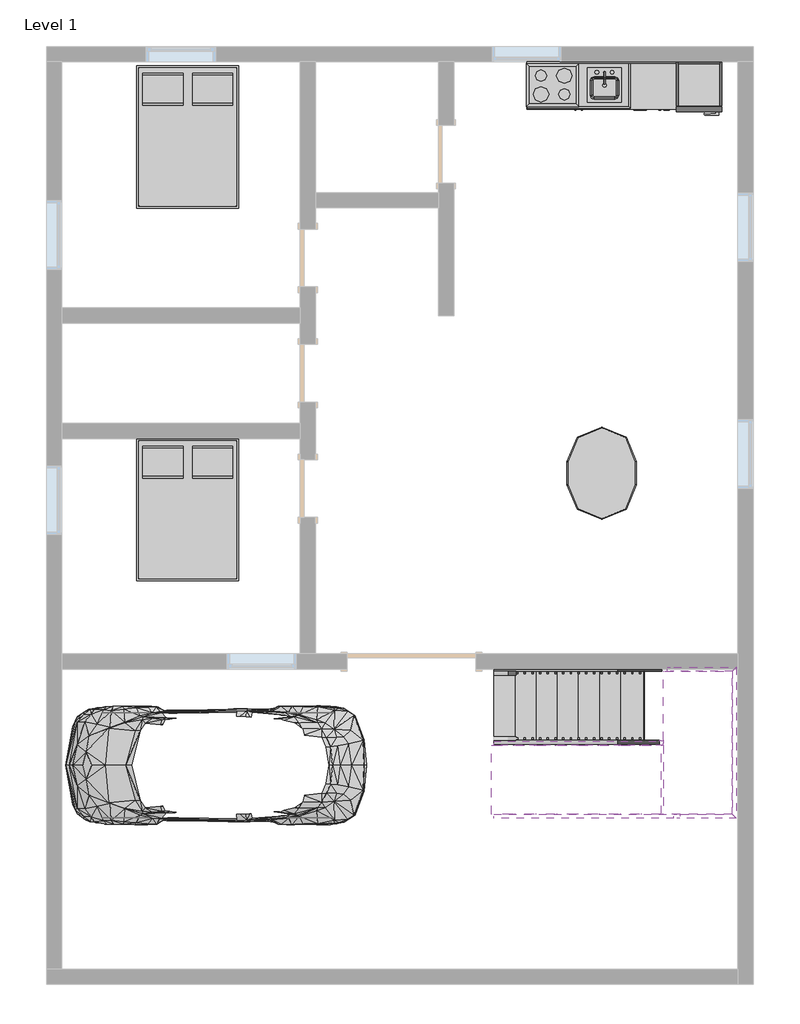
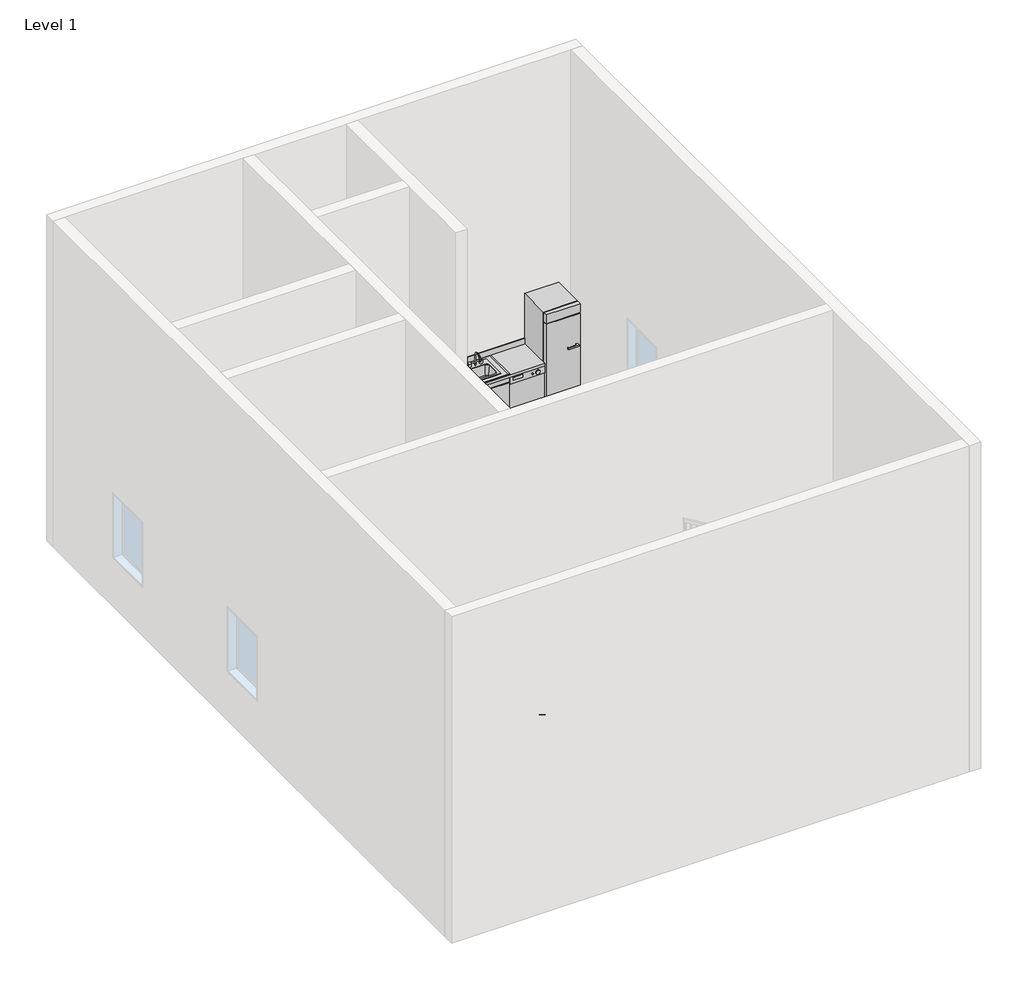
# One storey, part 2 of 2: 8 members, 5 proxies, 4 furniture elements, 2 stair flights, 1 flow terminal, 1 railing, 1 slab.
"""IFC4 building model written with IfcOpenShell, lengths in millimetres."""

from ifc_helpers import new_model, si_unit, frame, origin, place, context, project, spatial, polyline, outline, extrude, faceted_brep, transform, mapped, element, save
from components import m_cook_top_4_unit2_0615_x_500mm_249f3515, m_dishwasher_610_x_610_x_875mm_54ecfc4c, m_kitchenette_medium_1372mm_e05c6bec, m_rpc_beetle_m_rpc_beetle_aa710b07, m_refrigerator_600_x_660mm_a466bf94, m_sink_kitchen_island_450_x_450mm_f969cf2d, m_bed_box_1346_x_1880mm_double_b32eb57e, m_counter_top_w_sink_hole_600mm_depth_0a237b63, m_table_dining_oval_0915_x_1220mm_c3de6a6b, non_monolithic_landing_275f9134, stair_flight_1fa62499, stair_flight_e850d810

model = new_model("IFC4")

# Units and contexts
model_context = context("Model", 3, world=origin())
ifc_project = project(units=[si_unit("LENGTHUNIT", "METRE", prefix="MILLI")], contexts=[model_context])

# Site, building, storey
site = spatial("IfcSite", under=ifc_project)
building = spatial("IfcBuilding", under=site)
storey = spatial("IfcBuildingStorey", under=building, Name="Level 1", Elevation=0.0)

# Proxies
placement = place(None, origin())
m_cook_top_4_unit2_0615_x_500mm_shape = m_cook_top_4_unit2_0615_x_500mm_249f3515(model_context)
element("IfcBuildingElementProxy", 1, Name="M_Cook Top-4 Unit2 : 0615 x 500mm", ObjectType="M_Cook Top-4 Unit2 : 0615 x 500mm", at=placement, inside=storey, context=model_context, shape_type="MappedRepresentation", body=[
    mapped(m_cook_top_4_unit2_0615_x_500mm_shape, transform((-3150.6851125, 9903.2979873, 0.0), x_axis=(1.0, 0.0, 0.0), y_axis=(0.0, 1.0, 0.0), z_axis=(0.0, 0.0, 1.0))),
])
m_dishwasher_610_x_610_x_875mm_shape = m_dishwasher_610_x_610_x_875mm_54ecfc4c(model_context)
element("IfcBuildingElementProxy", 2, Name="M_Dishwasher : 610 x 610 x 875mm", ObjectType="M_Dishwasher : 610 x 610 x 875mm", at=placement, inside=storey, context=model_context, shape_type="MappedRepresentation", body=[
    mapped(m_dishwasher_610_x_610_x_875mm_shape, transform((-2201.202581, 9636.6484225, 0.0), x_axis=(1.0, 0.0, 0.0), y_axis=(0.0, 1.0, 0.0), z_axis=(0.0, 0.0, 1.0))),
])
m_kitchenette_medium_1372mm_shape = m_kitchenette_medium_1372mm_e05c6bec(model_context)
element("IfcBuildingElementProxy", 3, Name="M_Kitchenette - Medium : 1372mm", ObjectType="M_Kitchenette - Medium : 1372mm", at=placement, inside=storey, context=model_context, shape_type="MappedRepresentation", body=[
    mapped(m_kitchenette_medium_1372mm_shape, transform((-2826.4228174, 10208.2979873, 0.0), x_axis=(1.0, 0.0, 0.0), y_axis=(0.0, 1.0, 0.0), z_axis=(0.0, 0.0, 1.0))),
])
m_rpc_beetle_m_rpc_beetle_shape = m_rpc_beetle_m_rpc_beetle_aa710b07(model_context)
element("IfcBuildingElementProxy", 4, Name="M_RPC Beetle : M_RPC Beetle", ObjectType="M_RPC Beetle : M_RPC Beetle", at=placement, inside=storey, context=model_context, shape_type="MappedRepresentation", body=[
    mapped(m_rpc_beetle_m_rpc_beetle_shape, transform((-6363.8851125, 911.8979873, 0.0), x_axis=(0.0, 1.0000000000000002, 0.0), y_axis=(-1.0000000000000002, 0.0, 0.0), z_axis=(0.0, 0.0, 1.0))),
])
m_refrigerator_600_x_660mm_shape = m_refrigerator_600_x_660mm_a466bf94(model_context)
element("IfcBuildingElementProxy", 5, Name="M_Refrigerator : 600 x 660mm", ObjectType="M_Refrigerator : 600 x 660mm", at=placement, inside=storey, context=model_context, shape_type="MappedRepresentation", body=[
    mapped(m_refrigerator_600_x_660mm_shape, transform((-1159.8839698, 9912.0828971, 0.0), x_axis=(1.0, 0.0, 0.0), y_axis=(0.0, 1.0, 0.0), z_axis=(0.0, 0.0, 1.0))),
])

# Flow terminal
m_sink_kitchen_island_450_x_450mm_shape = m_sink_kitchen_island_450_x_450mm_f969cf2d(model_context)
element("IfcFlowTerminal", 6, ObjectType="M_Sink Kitchen-Island : 450 x 450mm", at=placement, inside=storey, context=model_context, shape_type="MappedRepresentation", body=[
    mapped(m_sink_kitchen_island_450_x_450mm_shape, transform((-2480.374353, 9900.9525861, 0.0), x_axis=(1.0, 0.0, 0.0), y_axis=(0.0, 1.0, 0.0), z_axis=(0.0, 0.0, 1.0))),
])

# Furniture
m_bed_box_1346_x_1880mm_double_shape = m_bed_box_1346_x_1880mm_double_b32eb57e(model_context)
element("IfcFurniture", 7, ObjectType="M_Bed-Box : 1346 x 1880mm - Double", at=placement, inside=storey, context=model_context, shape_type="MappedRepresentation", body=[
    mapped(m_bed_box_1346_x_1880mm_double_shape, transform((-8315.8375715, 9452.3274955, 0.0), x_axis=(1.0, 0.0, 0.0), y_axis=(0.0, 1.0, 0.0), z_axis=(0.0, 0.0, 1.0))),
])
element("IfcFurniture", 8, ObjectType="M_Bed-Box : 1346 x 1880mm - Double", at=placement, inside=storey, context=model_context, shape_type="MappedRepresentation", body=[
    mapped(m_bed_box_1346_x_1880mm_double_shape, transform((-8315.8375715, 4524.3274955, 0.0), x_axis=(1.0, 0.0, 0.0), y_axis=(0.0, 1.0, 0.0), z_axis=(0.0, 0.0, 1.0))),
])
m_counter_top_w_sink_hole_600mm_depth_shape = m_counter_top_w_sink_hole_600mm_depth_0a237b63(model_context)
element("IfcFurniture", 9, ObjectType="M_Counter Top w Sink Hole : 600mm Depth", at=placement, inside=storey, context=model_context, shape_type="MappedRepresentation", body=[
    mapped(m_counter_top_w_sink_hole_600mm_depth_shape, transform((-2293.2228174, 10208.2979873, 0.0), x_axis=(1.0, 0.0, 0.0), y_axis=(0.0, 1.0, 0.0), z_axis=(0.0, 0.0, 1.0))),
])
m_table_dining_oval_0915_x_1220mm_shape = m_table_dining_oval_0915_x_1220mm_c3de6a6b(model_context)
element("IfcFurniture", 10, ObjectType="M_Table-Dining Oval : 0915 x 1220mm", at=placement, inside=storey, context=model_context, shape_type="MappedRepresentation", body=[
    mapped(m_table_dining_oval_0915_x_1220mm_shape, transform((-2860.4834731, 5174.2176594, 0.0), x_axis=(0.0, 1.0000000000000002, 0.0), y_axis=(-1.0000000000000002, 0.0, 0.0), z_axis=(0.0, 0.0, 1.0))),
])

# Members
element("IfcMember", 11, ObjectType="Stringer - 2\" Width", at=placement, inside=storey, context=model_context, shape_type="SweptSolid", body=[
    extrude(outline(polyline([(212.114512, -3925.4851125), (0.0, -3925.4851125), (0.0, -3687.3996007), (1295.4, -1549.9896007), (1600.2, -1635.1440572), (212.114512, -3925.4851125)])), frame((0.0, 2156.5395264, 0.0), z_axis=(0.0, 1.0, 0.0), x_axis=(0.0, 0.0, 1.0)), (0.0, 0.0, 1.0), 50.8),
])
element("IfcMember", 12, ObjectType="Stringer - 2\" Width", at=placement, inside=storey, context=model_context, shape_type="SweptSolid", body=[
    extrude(outline(polyline([(212.114512, -3925.4851125), (0.0, -3925.4851125), (0.0, -3687.3996007), (1179.5845383, -1741.0851125), (1535.9932998, -1741.0851125), (212.114512, -3925.4851125)])), frame((0.0, 1191.3395264, 0.0), z_axis=(0.0, 1.0, 0.0), x_axis=(0.0, 0.0, 1.0)), (0.0, 0.0, 1.0), 50.8),
])
element("IfcMember", 13, ObjectType="Stringer - 2\" Width", at=placement, inside=storey, context=model_context, shape_type="SweptSolid", body=[
    extrude(outline(polyline([(1295.4, -1551.1806242), (1600.2, -1466.0261677), (3090.7811786, -3925.4851125), (2734.3724171, -3925.4851125), (1295.4, -1551.1806242)])), frame((0.0, 213.9428815, 0.0), z_axis=(0.0, 1.0, 0.0), x_axis=(0.0, 0.0, 1.0)), (0.0, 0.0, 1.0), 50.8),
])
element("IfcMember", 14, ObjectType="Stringer - 2\" Width", at=placement, inside=storey, context=model_context, shape_type="SweptSolid", body=[
    extrude(outline(polyline([(1379.7057504, -1690.2851125), (1736.114512, -1690.2851125), (3090.7811786, -3925.4851125), (2734.3724171, -3925.4851125), (1379.7057504, -1690.2851125)])), frame((0.0, 1179.1428815, 0.0), z_axis=(0.0, 1.0, 0.0), x_axis=(0.0, 0.0, 1.0)), (0.0, 0.0, 1.0), 50.8),
])
element("IfcMember", 15, ObjectType="Stringer - 2\" Width", at=placement, inside=storey, context=model_context, shape_type="Brep", body=[
    faceted_brep([(-1466.0261677, 264.7428815, 1600.2), (-1466.0261677, 213.9428815, 1600.2), (-725.0851125, 213.9428815, 1600.2), (-775.8851125, 264.7428815, 1600.2), (-1551.1806242, 264.7428815, 1295.4), (-775.8851125, 264.7428815, 1295.4), (-1551.1806242, 213.9428815, 1295.4), (-725.0851125, 213.9428815, 1295.4)], [[[0, 1, 2, 3]], [[4, 0, 3, 5]], [[6, 4, 5, 7]], [[1, 6, 7, 2]], [[1, 0, 4, 6]], [[2, 7, 5, 3]]]),
])
element("IfcMember", 16, ObjectType="Stringer - 2\" Width", at=placement, inside=storey, context=model_context, shape_type="SweptSolid", body=[
    extrude(outline(polyline([(-725.0851125, 213.9428815), (-775.8851125, 264.7428815), (-775.8851125, 2156.5395264), (-725.0851125, 2207.3395264), (-725.0851125, 213.9428815)])), frame((0.0, 0.0, 1295.4), z_axis=(0.0, 0.0, 1.0), x_axis=(1.0, 0.0, 0.0)), (0.0, 0.0, 1.0), 304.8),
])
element("IfcMember", 17, ObjectType="Stringer - 2\" Width", at=placement, inside=storey, context=model_context, shape_type="Brep", body=[
    faceted_brep([(-775.8851125, 2156.5395264, 1600.2), (-725.0851125, 2207.3395264, 1600.2), (-1635.1440572, 2207.3395264, 1600.2), (-1635.1440572, 2156.5395264, 1600.2), (-775.8851125, 2156.5395264, 1295.4), (-1549.9896007, 2156.5395264, 1295.4), (-725.0851125, 2207.3395264, 1295.4), (-1549.9896007, 2207.3395264, 1295.4)], [[[0, 1, 2, 3]], [[4, 0, 3, 5]], [[6, 4, 5, 7]], [[1, 6, 7, 2]], [[1, 0, 4, 6]], [[2, 7, 5, 3]]]),
])
element("IfcMember", 18, ObjectType="Stringer - 2\" Width", at=placement, inside=storey, context=model_context, shape_type="SweptSolid", body=[
    extrude(outline(polyline([(-1741.0851125, 1242.1395264), (-1690.2851125, 1242.1395264), (-1690.2851125, 1229.9428815), (-1741.0851125, 1229.9428815), (-1741.0851125, 1242.1395264)])), frame((0.0, 0.0, 1295.4), z_axis=(0.0, 0.0, 1.0), x_axis=(1.0, 0.0, 0.0)), (0.0, 0.0, 1.0), 304.8),
])

# Railing
element("IfcRailing", 19, ObjectType="Handrail - Rectangular", at=placement, inside=storey, context=model_context, shape_type="SolidModel", body=[
    faceted_brep([(-3925.4851125, 2156.5395264, 1083.7333333), (-3925.4851125, 2156.5395264, 1024.3318731), (-3925.4851125, 2105.7395264, 1024.3318731), (-3925.4851125, 2105.7395264, 1083.7333333), (-1690.2851125, 2156.5395264, 2438.4), (-1676.0927031, 2156.5395264, 2387.6), (-1676.0927031, 2105.7395264, 2387.6), (-1690.2851125, 2105.7395264, 2438.4), (-775.8851125, 2156.5395264, 2438.4), (-775.8851125, 2156.5395264, 2387.6), (-826.6851125, 2105.7395264, 2387.6), (-826.6851125, 2105.7395264, 2438.4), (-775.8851125, 264.7428815, 2438.4), (-775.8851125, 264.7428815, 2387.6), (-826.6851125, 315.5428815, 2387.6), (-826.6851125, 315.5428815, 2438.4), (-1410.8851125, 264.7428815, 2438.4), (-1425.0775219, 264.7428815, 2387.6), (-1425.0775219, 315.5428815, 2387.6), (-1410.8851125, 315.5428815, 2438.4), (-3925.4851125, 264.7428815, 3962.4), (-3925.4851125, 315.5428815, 3962.4), (-3925.4851125, 315.5428815, 3902.9985397), (-3925.4851125, 264.7428815, 3902.9985397)], [[[0, 1, 2, 3]], [[1, 0, 4, 5]], [[2, 1, 5, 6]], [[3, 2, 6, 7]], [[0, 3, 7, 4]], [[5, 4, 8, 9]], [[6, 5, 9, 10]], [[7, 6, 10, 11]], [[4, 7, 11, 8]], [[9, 8, 12, 13]], [[10, 9, 13, 14]], [[11, 10, 14, 15]], [[8, 11, 15, 12]], [[13, 12, 16, 17]], [[14, 13, 17, 18]], [[15, 14, 18, 19]], [[12, 15, 19, 16]], [[20, 21, 22, 23]], [[17, 16, 20, 23]], [[18, 17, 23, 22]], [[19, 18, 22, 21]], [[16, 19, 21, 20]]]),
    extrude(outline(polyline([(3862.5894488, -3858.8101125), (2878.6666667, -3858.8101125), (2878.6666667, -3839.7601125), (3851.0439943, -3839.7601125), (3862.5894488, -3858.8101125)])), frame((0.0, 280.6178815, 0.0), z_axis=(0.0, 1.0, 0.0), x_axis=(0.0, 0.0, 1.0)), (0.0, 0.0, 1.0), 19.05),
    extrude(outline(polyline([(3801.0136913, -3757.2101125), (2878.6666667, -3757.2101125), (2878.6666667, -3738.1601125), (3789.4682367, -3738.1601125), (3801.0136913, -3757.2101125)])), frame((0.0, 280.6178815, 0.0), z_axis=(0.0, 1.0, 0.0), x_axis=(0.0, 0.0, 1.0)), (0.0, 0.0, 1.0), 19.05),
    extrude(outline(polyline([(3739.4379337, -3655.6101125), (2878.6666667, -3655.6101125), (2878.6666667, -3636.5601125), (3727.8924791, -3636.5601125), (3739.4379337, -3655.6101125)])), frame((0.0, 280.6178815, 0.0), z_axis=(0.0, 1.0, 0.0), x_axis=(0.0, 0.0, 1.0)), (0.0, 0.0, 1.0), 19.05),
    extrude(outline(polyline([(3677.8621761, -3554.0101125), (2709.3333333, -3554.0101125), (2709.3333333, -3534.9601125), (3666.3167216, -3534.9601125), (3677.8621761, -3554.0101125)])), frame((0.0, 280.6178815, 0.0), z_axis=(0.0, 1.0, 0.0), x_axis=(0.0, 0.0, 1.0)), (0.0, 0.0, 1.0), 19.05),
    extrude(outline(polyline([(3616.2864185, -3452.4101125), (2709.3333333, -3452.4101125), (2709.3333333, -3433.3601125), (3604.740964, -3433.3601125), (3616.2864185, -3452.4101125)])), frame((0.0, 280.6178815, 0.0), z_axis=(0.0, 1.0, 0.0), x_axis=(0.0, 0.0, 1.0)), (0.0, 0.0, 1.0), 19.05),
    extrude(outline(polyline([(3554.710661, -3350.8101125), (2540.0, -3350.8101125), (2540.0, -3331.7601125), (3543.1652064, -3331.7601125), (3554.710661, -3350.8101125)])), frame((0.0, 280.6178815, 0.0), z_axis=(0.0, 1.0, 0.0), x_axis=(0.0, 0.0, 1.0)), (0.0, 0.0, 1.0), 19.05),
    extrude(outline(polyline([(3493.1349034, -3249.2101125), (2540.0, -3249.2101125), (2540.0, -3230.1601125), (3481.5894488, -3230.1601125), (3493.1349034, -3249.2101125)])), frame((0.0, 280.6178815, 0.0), z_axis=(0.0, 1.0, 0.0), x_axis=(0.0, 0.0, 1.0)), (0.0, 0.0, 1.0), 19.05),
    extrude(outline(polyline([(3431.5591458, -3147.6101125), (2540.0, -3147.6101125), (2540.0, -3128.5601125), (3420.0136913, -3128.5601125), (3431.5591458, -3147.6101125)])), frame((0.0, 280.6178815, 0.0), z_axis=(0.0, 1.0, 0.0), x_axis=(0.0, 0.0, 1.0)), (0.0, 0.0, 1.0), 19.05),
    extrude(outline(polyline([(3369.9833882, -3046.0101125), (2370.6666667, -3046.0101125), (2370.6666667, -3026.9601125), (3358.4379337, -3026.9601125), (3369.9833882, -3046.0101125)])), frame((0.0, 280.6178815, 0.0), z_axis=(0.0, 1.0, 0.0), x_axis=(0.0, 0.0, 1.0)), (0.0, 0.0, 1.0), 19.05),
    extrude(outline(polyline([(3308.4076307, -2944.4101125), (2370.6666667, -2944.4101125), (2370.6666667, -2925.3601125), (3296.8621761, -2925.3601125), (3308.4076307, -2944.4101125)])), frame((0.0, 280.6178815, 0.0), z_axis=(0.0, 1.0, 0.0), x_axis=(0.0, 0.0, 1.0)), (0.0, 0.0, 1.0), 19.05),
    extrude(outline(polyline([(3246.8318731, -2842.8101125), (2370.6666667, -2842.8101125), (2370.6666667, -2823.7601125), (3235.2864185, -2823.7601125), (3246.8318731, -2842.8101125)])), frame((0.0, 280.6178815, 0.0), z_axis=(0.0, 1.0, 0.0), x_axis=(0.0, 0.0, 1.0)), (0.0, 0.0, 1.0), 19.05),
    extrude(outline(polyline([(3185.2561155, -2741.2101125), (2201.3333333, -2741.2101125), (2201.3333333, -2722.1601125), (3173.710661, -2722.1601125), (3185.2561155, -2741.2101125)])), frame((0.0, 280.6178815, 0.0), z_axis=(0.0, 1.0, 0.0), x_axis=(0.0, 0.0, 1.0)), (0.0, 0.0, 1.0), 19.05),
    extrude(outline(polyline([(3123.6803579, -2639.6101125), (2201.3333333, -2639.6101125), (2201.3333333, -2620.5601125), (3112.1349034, -2620.5601125), (3123.6803579, -2639.6101125)])), frame((0.0, 280.6178815, 0.0), z_axis=(0.0, 1.0, 0.0), x_axis=(0.0, 0.0, 1.0)), (0.0, 0.0, 1.0), 19.05),
    extrude(outline(polyline([(3062.1046004, -2538.0101125), (2201.3333333, -2538.0101125), (2201.3333333, -2518.9601125), (3050.5591458, -2518.9601125), (3062.1046004, -2538.0101125)])), frame((0.0, 280.6178815, 0.0), z_axis=(0.0, 1.0, 0.0), x_axis=(0.0, 0.0, 1.0)), (0.0, 0.0, 1.0), 19.05),
    extrude(outline(polyline([(3000.5288428, -2436.4101125), (2032.0, -2436.4101125), (2032.0, -2417.3601125), (2988.9833882, -2417.3601125), (3000.5288428, -2436.4101125)])), frame((0.0, 280.6178815, 0.0), z_axis=(0.0, 1.0, 0.0), x_axis=(0.0, 0.0, 1.0)), (0.0, 0.0, 1.0), 19.05),
    extrude(outline(polyline([(2938.9530852, -2334.8101125), (2032.0, -2334.8101125), (2032.0, -2315.7601125), (2927.4076307, -2315.7601125), (2938.9530852, -2334.8101125)])), frame((0.0, 280.6178815, 0.0), z_axis=(0.0, 1.0, 0.0), x_axis=(0.0, 0.0, 1.0)), (0.0, 0.0, 1.0), 19.05),
    extrude(outline(polyline([(2877.3773276, -2233.2101125), (1862.6666667, -2233.2101125), (1862.6666667, -2214.1601125), (2865.8318731, -2214.1601125), (2877.3773276, -2233.2101125)])), frame((0.0, 280.6178815, 0.0), z_axis=(0.0, 1.0, 0.0), x_axis=(0.0, 0.0, 1.0)), (0.0, 0.0, 1.0), 19.05),
    extrude(outline(polyline([(2815.80157, -2131.6101125), (1862.6666667, -2131.6101125), (1862.6666667, -2112.5601125), (2804.2561155, -2112.5601125), (2815.80157, -2131.6101125)])), frame((0.0, 280.6178815, 0.0), z_axis=(0.0, 1.0, 0.0), x_axis=(0.0, 0.0, 1.0)), (0.0, 0.0, 1.0), 19.05),
    extrude(outline(polyline([(2754.2258125, -2030.0101125), (1862.6666667, -2030.0101125), (1862.6666667, -2010.9601125), (2742.6803579, -2010.9601125), (2754.2258125, -2030.0101125)])), frame((0.0, 280.6178815, 0.0), z_axis=(0.0, 1.0, 0.0), x_axis=(0.0, 0.0, 1.0)), (0.0, 0.0, 1.0), 19.05),
    extrude(outline(polyline([(2692.6500549, -1928.4101125), (1693.3333333, -1928.4101125), (1693.3333333, -1909.3601125), (2681.1046004, -1909.3601125), (2692.6500549, -1928.4101125)])), frame((0.0, 280.6178815, 0.0), z_axis=(0.0, 1.0, 0.0), x_axis=(0.0, 0.0, 1.0)), (0.0, 0.0, 1.0), 19.05),
    extrude(outline(polyline([(2631.0742973, -1826.8101125), (1693.3333333, -1826.8101125), (1693.3333333, -1807.7601125), (2619.5288428, -1807.7601125), (2631.0742973, -1826.8101125)])), frame((0.0, 280.6178815, 0.0), z_axis=(0.0, 1.0, 0.0), x_axis=(0.0, 0.0, 1.0)), (0.0, 0.0, 1.0), 19.05),
    extrude(outline(polyline([(2569.4985397, -1725.2101125), (1693.3333333, -1725.2101125), (1693.3333333, -1706.1601125), (2557.9530852, -1706.1601125), (2569.4985397, -1725.2101125)])), frame((0.0, 280.6178815, 0.0), z_axis=(0.0, 1.0, 0.0), x_axis=(0.0, 0.0, 1.0)), (0.0, 0.0, 1.0), 19.05),
    extrude(outline(polyline([(2507.9227822, -1623.6101125), (1524.0, -1623.6101125), (1524.0, -1604.5601125), (2496.3773276, -1604.5601125), (2507.9227822, -1623.6101125)])), frame((0.0, 280.6178815, 0.0), z_axis=(0.0, 1.0, 0.0), x_axis=(0.0, 0.0, 1.0)), (0.0, 0.0, 1.0), 19.05),
    extrude(outline(polyline([(2446.3470246, -1522.0101125), (1524.0, -1522.0101125), (1524.0, -1502.9601125), (2434.80157, -1502.9601125), (2446.3470246, -1522.0101125)])), frame((0.0, 280.6178815, 0.0), z_axis=(0.0, 1.0, 0.0), x_axis=(0.0, 0.0, 1.0)), (0.0, 0.0, 1.0), 19.05),
    extrude(outline(polyline([(-1299.7601125, 280.6178815), (-1318.8101125, 280.6178815), (-1318.8101125, 299.6678815), (-1299.7601125, 299.6678815), (-1299.7601125, 280.6178815)])), frame((0.0, 0.0, 1524.0), z_axis=(0.0, 0.0, 1.0), x_axis=(1.0, 0.0, 0.0)), (0.0, 0.0, 1.0), 863.6),
    extrude(outline(polyline([(-1198.1601125, 280.6178815), (-1217.2101125, 280.6178815), (-1217.2101125, 299.6678815), (-1198.1601125, 299.6678815), (-1198.1601125, 280.6178815)])), frame((0.0, 0.0, 1524.0), z_axis=(0.0, 0.0, 1.0), x_axis=(1.0, 0.0, 0.0)), (0.0, 0.0, 1.0), 863.6),
    extrude(outline(polyline([(-1096.5601125, 280.6178815), (-1115.6101125, 280.6178815), (-1115.6101125, 299.6678815), (-1096.5601125, 299.6678815), (-1096.5601125, 280.6178815)])), frame((0.0, 0.0, 1524.0), z_axis=(0.0, 0.0, 1.0), x_axis=(1.0, 0.0, 0.0)), (0.0, 0.0, 1.0), 863.6),
    extrude(outline(polyline([(-994.9601125, 280.6178815), (-1014.0101125, 280.6178815), (-1014.0101125, 299.6678815), (-994.9601125, 299.6678815), (-994.9601125, 280.6178815)])), frame((0.0, 0.0, 1524.0), z_axis=(0.0, 0.0, 1.0), x_axis=(1.0, 0.0, 0.0)), (0.0, 0.0, 1.0), 863.6),
    extrude(outline(polyline([(-893.3601125, 280.6178815), (-912.4101125, 280.6178815), (-912.4101125, 299.6678815), (-893.3601125, 299.6678815), (-893.3601125, 280.6178815)])), frame((0.0, 0.0, 1524.0), z_axis=(0.0, 0.0, 1.0), x_axis=(1.0, 0.0, 0.0)), (0.0, 0.0, 1.0), 863.6),
    extrude(outline(polyline([(-791.7601125, 311.8645264), (-791.7601125, 292.8145264), (-810.8101125, 292.8145264), (-810.8101125, 311.8645264), (-791.7601125, 311.8645264)])), frame((0.0, 0.0, 1524.0), z_axis=(0.0, 0.0, 1.0), x_axis=(1.0, 0.0, 0.0)), (0.0, 0.0, 1.0), 863.6),
    extrude(outline(polyline([(-791.7601125, 413.4645264), (-791.7601125, 394.4145264), (-810.8101125, 394.4145264), (-810.8101125, 413.4645264), (-791.7601125, 413.4645264)])), frame((0.0, 0.0, 1524.0), z_axis=(0.0, 0.0, 1.0), x_axis=(1.0, 0.0, 0.0)), (0.0, 0.0, 1.0), 863.6),
    extrude(outline(polyline([(-791.7601125, 515.0645264), (-791.7601125, 496.0145264), (-810.8101125, 496.0145264), (-810.8101125, 515.0645264), (-791.7601125, 515.0645264)])), frame((0.0, 0.0, 1524.0), z_axis=(0.0, 0.0, 1.0), x_axis=(1.0, 0.0, 0.0)), (0.0, 0.0, 1.0), 863.6),
    extrude(outline(polyline([(-791.7601125, 616.6645264), (-791.7601125, 597.6145264), (-810.8101125, 597.6145264), (-810.8101125, 616.6645264), (-791.7601125, 616.6645264)])), frame((0.0, 0.0, 1524.0), z_axis=(0.0, 0.0, 1.0), x_axis=(1.0, 0.0, 0.0)), (0.0, 0.0, 1.0), 863.6),
    extrude(outline(polyline([(-791.7601125, 718.2645264), (-791.7601125, 699.2145264), (-810.8101125, 699.2145264), (-810.8101125, 718.2645264), (-791.7601125, 718.2645264)])), frame((0.0, 0.0, 1524.0), z_axis=(0.0, 0.0, 1.0), x_axis=(1.0, 0.0, 0.0)), (0.0, 0.0, 1.0), 863.6),
    extrude(outline(polyline([(-791.7601125, 819.8645264), (-791.7601125, 800.8145264), (-810.8101125, 800.8145264), (-810.8101125, 819.8645264), (-791.7601125, 819.8645264)])), frame((0.0, 0.0, 1524.0), z_axis=(0.0, 0.0, 1.0), x_axis=(1.0, 0.0, 0.0)), (0.0, 0.0, 1.0), 863.6),
    extrude(outline(polyline([(-791.7601125, 921.4645264), (-791.7601125, 902.4145264), (-810.8101125, 902.4145264), (-810.8101125, 921.4645264), (-791.7601125, 921.4645264)])), frame((0.0, 0.0, 1524.0), z_axis=(0.0, 0.0, 1.0), x_axis=(1.0, 0.0, 0.0)), (0.0, 0.0, 1.0), 863.6),
    extrude(outline(polyline([(-791.7601125, 1023.0645264), (-791.7601125, 1004.0145264), (-810.8101125, 1004.0145264), (-810.8101125, 1023.0645264), (-791.7601125, 1023.0645264)])), frame((0.0, 0.0, 1524.0), z_axis=(0.0, 0.0, 1.0), x_axis=(1.0, 0.0, 0.0)), (0.0, 0.0, 1.0), 863.6),
    extrude(outline(polyline([(-791.7601125, 1124.6645264), (-791.7601125, 1105.6145264), (-810.8101125, 1105.6145264), (-810.8101125, 1124.6645264), (-791.7601125, 1124.6645264)])), frame((0.0, 0.0, 1524.0), z_axis=(0.0, 0.0, 1.0), x_axis=(1.0, 0.0, 0.0)), (0.0, 0.0, 1.0), 863.6),
    extrude(outline(polyline([(-791.7601125, 1226.2645264), (-791.7601125, 1207.2145264), (-810.8101125, 1207.2145264), (-810.8101125, 1226.2645264), (-791.7601125, 1226.2645264)])), frame((0.0, 0.0, 1524.0), z_axis=(0.0, 0.0, 1.0), x_axis=(1.0, 0.0, 0.0)), (0.0, 0.0, 1.0), 863.6),
    extrude(outline(polyline([(-791.7601125, 1327.8645264), (-791.7601125, 1308.8145264), (-810.8101125, 1308.8145264), (-810.8101125, 1327.8645264), (-791.7601125, 1327.8645264)])), frame((0.0, 0.0, 1524.0), z_axis=(0.0, 0.0, 1.0), x_axis=(1.0, 0.0, 0.0)), (0.0, 0.0, 1.0), 863.6),
    extrude(outline(polyline([(-791.7601125, 1429.4645264), (-791.7601125, 1410.4145264), (-810.8101125, 1410.4145264), (-810.8101125, 1429.4645264), (-791.7601125, 1429.4645264)])), frame((0.0, 0.0, 1524.0), z_axis=(0.0, 0.0, 1.0), x_axis=(1.0, 0.0, 0.0)), (0.0, 0.0, 1.0), 863.6),
    extrude(outline(polyline([(-791.7601125, 1531.0645264), (-791.7601125, 1512.0145264), (-810.8101125, 1512.0145264), (-810.8101125, 1531.0645264), (-791.7601125, 1531.0645264)])), frame((0.0, 0.0, 1524.0), z_axis=(0.0, 0.0, 1.0), x_axis=(1.0, 0.0, 0.0)), (0.0, 0.0, 1.0), 863.6),
    extrude(outline(polyline([(-791.7601125, 1632.6645264), (-791.7601125, 1613.6145264), (-810.8101125, 1613.6145264), (-810.8101125, 1632.6645264), (-791.7601125, 1632.6645264)])), frame((0.0, 0.0, 1524.0), z_axis=(0.0, 0.0, 1.0), x_axis=(1.0, 0.0, 0.0)), (0.0, 0.0, 1.0), 863.6),
    extrude(outline(polyline([(-791.7601125, 1734.2645264), (-791.7601125, 1715.2145264), (-810.8101125, 1715.2145264), (-810.8101125, 1734.2645264), (-791.7601125, 1734.2645264)])), frame((0.0, 0.0, 1524.0), z_axis=(0.0, 0.0, 1.0), x_axis=(1.0, 0.0, 0.0)), (0.0, 0.0, 1.0), 863.6),
    extrude(outline(polyline([(-791.7601125, 1835.8645264), (-791.7601125, 1816.8145264), (-810.8101125, 1816.8145264), (-810.8101125, 1835.8645264), (-791.7601125, 1835.8645264)])), frame((0.0, 0.0, 1524.0), z_axis=(0.0, 0.0, 1.0), x_axis=(1.0, 0.0, 0.0)), (0.0, 0.0, 1.0), 863.6),
    extrude(outline(polyline([(-791.7601125, 1937.4645264), (-791.7601125, 1918.4145264), (-810.8101125, 1918.4145264), (-810.8101125, 1937.4645264), (-791.7601125, 1937.4645264)])), frame((0.0, 0.0, 1524.0), z_axis=(0.0, 0.0, 1.0), x_axis=(1.0, 0.0, 0.0)), (0.0, 0.0, 1.0), 863.6),
    extrude(outline(polyline([(-791.7601125, 2039.0645264), (-791.7601125, 2020.0145264), (-810.8101125, 2020.0145264), (-810.8101125, 2039.0645264), (-791.7601125, 2039.0645264)])), frame((0.0, 0.0, 1524.0), z_axis=(0.0, 0.0, 1.0), x_axis=(1.0, 0.0, 0.0)), (0.0, 0.0, 1.0), 863.6),
    extrude(outline(polyline([(-887.0101125, 2140.6645264), (-867.9601125, 2140.6645264), (-867.9601125, 2121.6145264), (-887.0101125, 2121.6145264), (-887.0101125, 2140.6645264)])), frame((0.0, 0.0, 1524.0), z_axis=(0.0, 0.0, 1.0), x_axis=(1.0, 0.0, 0.0)), (0.0, 0.0, 1.0), 863.6),
    extrude(outline(polyline([(-988.6101125, 2140.6645264), (-969.5601125, 2140.6645264), (-969.5601125, 2121.6145264), (-988.6101125, 2121.6145264), (-988.6101125, 2140.6645264)])), frame((0.0, 0.0, 1524.0), z_axis=(0.0, 0.0, 1.0), x_axis=(1.0, 0.0, 0.0)), (0.0, 0.0, 1.0), 863.6),
    extrude(outline(polyline([(-1090.2101125, 2140.6645264), (-1071.1601125, 2140.6645264), (-1071.1601125, 2121.6145264), (-1090.2101125, 2121.6145264), (-1090.2101125, 2140.6645264)])), frame((0.0, 0.0, 1524.0), z_axis=(0.0, 0.0, 1.0), x_axis=(1.0, 0.0, 0.0)), (0.0, 0.0, 1.0), 863.6),
    extrude(outline(polyline([(-1191.8101125, 2140.6645264), (-1172.7601125, 2140.6645264), (-1172.7601125, 2121.6145264), (-1191.8101125, 2121.6145264), (-1191.8101125, 2140.6645264)])), frame((0.0, 0.0, 1524.0), z_axis=(0.0, 0.0, 1.0), x_axis=(1.0, 0.0, 0.0)), (0.0, 0.0, 1.0), 863.6),
    extrude(outline(polyline([(-1293.4101125, 2140.6645264), (-1274.3601125, 2140.6645264), (-1274.3601125, 2121.6145264), (-1293.4101125, 2121.6145264), (-1293.4101125, 2140.6645264)])), frame((0.0, 0.0, 1524.0), z_axis=(0.0, 0.0, 1.0), x_axis=(1.0, 0.0, 0.0)), (0.0, 0.0, 1.0), 863.6),
    extrude(outline(polyline([(-1395.0101125, 2140.6645264), (-1375.9601125, 2140.6645264), (-1375.9601125, 2121.6145264), (-1395.0101125, 2121.6145264), (-1395.0101125, 2140.6645264)])), frame((0.0, 0.0, 1524.0), z_axis=(0.0, 0.0, 1.0), x_axis=(1.0, 0.0, 0.0)), (0.0, 0.0, 1.0), 863.6),
    extrude(outline(polyline([(-1496.6101125, 2140.6645264), (-1477.5601125, 2140.6645264), (-1477.5601125, 2121.6145264), (-1496.6101125, 2121.6145264), (-1496.6101125, 2140.6645264)])), frame((0.0, 0.0, 1524.0), z_axis=(0.0, 0.0, 1.0), x_axis=(1.0, 0.0, 0.0)), (0.0, 0.0, 1.0), 863.6),
    extrude(outline(polyline([(-1598.2101125, 2140.6645264), (-1579.1601125, 2140.6645264), (-1579.1601125, 2121.6145264), (-1598.2101125, 2121.6145264), (-1598.2101125, 2140.6645264)])), frame((0.0, 0.0, 1524.0), z_axis=(0.0, 0.0, 1.0), x_axis=(1.0, 0.0, 0.0)), (0.0, 0.0, 1.0), 863.6),
    extrude(outline(polyline([(2311.6500549, -1801.4101125), (1354.6666667, -1801.4101125), (1354.6666667, -1782.3601125), (2323.1955094, -1782.3601125), (2311.6500549, -1801.4101125)])), frame((0.0, 2121.6145264, 0.0), z_axis=(0.0, 1.0, 0.0), x_axis=(0.0, 0.0, 1.0)), (0.0, 0.0, 1.0), 19.05),
    extrude(outline(polyline([(2250.0742973, -1903.0101125), (1354.6666667, -1903.0101125), (1354.6666667, -1883.9601125), (2261.6197519, -1883.9601125), (2250.0742973, -1903.0101125)])), frame((0.0, 2121.6145264, 0.0), z_axis=(0.0, 1.0, 0.0), x_axis=(0.0, 0.0, 1.0)), (0.0, 0.0, 1.0), 19.05),
    extrude(outline(polyline([(2188.4985397, -2004.6101125), (1185.3333333, -2004.6101125), (1185.3333333, -1985.5601125), (2200.0439943, -1985.5601125), (2188.4985397, -2004.6101125)])), frame((0.0, 2121.6145264, 0.0), z_axis=(0.0, 1.0, 0.0), x_axis=(0.0, 0.0, 1.0)), (0.0, 0.0, 1.0), 19.05),
    extrude(outline(polyline([(2126.9227822, -2106.2101125), (1185.3333333, -2106.2101125), (1185.3333333, -2087.1601125), (2138.4682367, -2087.1601125), (2126.9227822, -2106.2101125)])), frame((0.0, 2121.6145264, 0.0), z_axis=(0.0, 1.0, 0.0), x_axis=(0.0, 0.0, 1.0)), (0.0, 0.0, 1.0), 19.05),
    extrude(outline(polyline([(2065.3470246, -2207.8101125), (1185.3333333, -2207.8101125), (1185.3333333, -2188.7601125), (2076.8924791, -2188.7601125), (2065.3470246, -2207.8101125)])), frame((0.0, 2121.6145264, 0.0), z_axis=(0.0, 1.0, 0.0), x_axis=(0.0, 0.0, 1.0)), (0.0, 0.0, 1.0), 19.05),
    extrude(outline(polyline([(2003.771267, -2309.4101125), (1016.0, -2309.4101125), (1016.0, -2290.3601125), (2015.3167216, -2290.3601125), (2003.771267, -2309.4101125)])), frame((0.0, 2121.6145264, 0.0), z_axis=(0.0, 1.0, 0.0), x_axis=(0.0, 0.0, 1.0)), (0.0, 0.0, 1.0), 19.05),
    extrude(outline(polyline([(1942.1955094, -2411.0101125), (1016.0, -2411.0101125), (1016.0, -2391.9601125), (1953.740964, -2391.9601125), (1942.1955094, -2411.0101125)])), frame((0.0, 2121.6145264, 0.0), z_axis=(0.0, 1.0, 0.0), x_axis=(0.0, 0.0, 1.0)), (0.0, 0.0, 1.0), 19.05),
    extrude(outline(polyline([(1880.6197519, -2512.6101125), (1016.0, -2512.6101125), (1016.0, -2493.5601125), (1892.1652064, -2493.5601125), (1880.6197519, -2512.6101125)])), frame((0.0, 2121.6145264, 0.0), z_axis=(0.0, 1.0, 0.0), x_axis=(0.0, 0.0, 1.0)), (0.0, 0.0, 1.0), 19.05),
    extrude(outline(polyline([(1819.0439943, -2614.2101125), (846.6666667, -2614.2101125), (846.6666667, -2595.1601125), (1830.5894488, -2595.1601125), (1819.0439943, -2614.2101125)])), frame((0.0, 2121.6145264, 0.0), z_axis=(0.0, 1.0, 0.0), x_axis=(0.0, 0.0, 1.0)), (0.0, 0.0, 1.0), 19.05),
    extrude(outline(polyline([(1757.4682367, -2715.8101125), (846.6666667, -2715.8101125), (846.6666667, -2696.7601125), (1769.0136913, -2696.7601125), (1757.4682367, -2715.8101125)])), frame((0.0, 2121.6145264, 0.0), z_axis=(0.0, 1.0, 0.0), x_axis=(0.0, 0.0, 1.0)), (0.0, 0.0, 1.0), 19.05),
    extrude(outline(polyline([(1695.8924791, -2817.4101125), (846.6666667, -2817.4101125), (846.6666667, -2798.3601125), (1707.4379337, -2798.3601125), (1695.8924791, -2817.4101125)])), frame((0.0, 2121.6145264, 0.0), z_axis=(0.0, 1.0, 0.0), x_axis=(0.0, 0.0, 1.0)), (0.0, 0.0, 1.0), 19.05),
    extrude(outline(polyline([(1634.3167216, -2919.0101125), (677.3333333, -2919.0101125), (677.3333333, -2899.9601125), (1645.8621761, -2899.9601125), (1634.3167216, -2919.0101125)])), frame((0.0, 2121.6145264, 0.0), z_axis=(0.0, 1.0, 0.0), x_axis=(0.0, 0.0, 1.0)), (0.0, 0.0, 1.0), 19.05),
    extrude(outline(polyline([(1572.740964, -3020.6101125), (677.3333333, -3020.6101125), (677.3333333, -3001.5601125), (1584.2864185, -3001.5601125), (1572.740964, -3020.6101125)])), frame((0.0, 2121.6145264, 0.0), z_axis=(0.0, 1.0, 0.0), x_axis=(0.0, 0.0, 1.0)), (0.0, 0.0, 1.0), 19.05),
    extrude(outline(polyline([(1511.1652064, -3122.2101125), (508.0, -3122.2101125), (508.0, -3103.1601125), (1522.710661, -3103.1601125), (1511.1652064, -3122.2101125)])), frame((0.0, 2121.6145264, 0.0), z_axis=(0.0, 1.0, 0.0), x_axis=(0.0, 0.0, 1.0)), (0.0, 0.0, 1.0), 19.05),
    extrude(outline(polyline([(1449.5894488, -3223.8101125), (508.0, -3223.8101125), (508.0, -3204.7601125), (1461.1349034, -3204.7601125), (1449.5894488, -3223.8101125)])), frame((0.0, 2121.6145264, 0.0), z_axis=(0.0, 1.0, 0.0), x_axis=(0.0, 0.0, 1.0)), (0.0, 0.0, 1.0), 19.05),
    extrude(outline(polyline([(1388.0136913, -3325.4101125), (508.0, -3325.4101125), (508.0, -3306.3601125), (1399.5591458, -3306.3601125), (1388.0136913, -3325.4101125)])), frame((0.0, 2121.6145264, 0.0), z_axis=(0.0, 1.0, 0.0), x_axis=(0.0, 0.0, 1.0)), (0.0, 0.0, 1.0), 19.05),
    extrude(outline(polyline([(1326.4379337, -3427.0101125), (338.6666667, -3427.0101125), (338.6666667, -3407.9601125), (1337.9833882, -3407.9601125), (1326.4379337, -3427.0101125)])), frame((0.0, 2121.6145264, 0.0), z_axis=(0.0, 1.0, 0.0), x_axis=(0.0, 0.0, 1.0)), (0.0, 0.0, 1.0), 19.05),
    extrude(outline(polyline([(1264.8621761, -3528.6101125), (338.6666667, -3528.6101125), (338.6666667, -3509.5601125), (1276.4076307, -3509.5601125), (1264.8621761, -3528.6101125)])), frame((0.0, 2121.6145264, 0.0), z_axis=(0.0, 1.0, 0.0), x_axis=(0.0, 0.0, 1.0)), (0.0, 0.0, 1.0), 19.05),
    extrude(outline(polyline([(1203.2864185, -3630.2101125), (338.6666667, -3630.2101125), (338.6666667, -3611.1601125), (1214.8318731, -3611.1601125), (1203.2864185, -3630.2101125)])), frame((0.0, 2121.6145264, 0.0), z_axis=(0.0, 1.0, 0.0), x_axis=(0.0, 0.0, 1.0)), (0.0, 0.0, 1.0), 19.05),
    extrude(outline(polyline([(1141.710661, -3731.8101125), (169.3333333, -3731.8101125), (169.3333333, -3712.7601125), (1153.2561155, -3712.7601125), (1141.710661, -3731.8101125)])), frame((0.0, 2121.6145264, 0.0), z_axis=(0.0, 1.0, 0.0), x_axis=(0.0, 0.0, 1.0)), (0.0, 0.0, 1.0), 19.05),
    extrude(outline(polyline([(1080.1349034, -3833.4101125), (169.3333333, -3833.4101125), (169.3333333, -3814.3601125), (1091.6803579, -3814.3601125), (1080.1349034, -3833.4101125)])), frame((0.0, 2121.6145264, 0.0), z_axis=(0.0, 1.0, 0.0), x_axis=(0.0, 0.0, 1.0)), (0.0, 0.0, 1.0), 19.05),
    extrude(outline(polyline([(-1401.3601125, 280.6178815), (-1420.4101125, 280.6178815), (-1420.4101125, 299.6678815), (-1401.3601125, 299.6678815), (-1401.3601125, 280.6178815)])), frame((0.0, 0.0, 1524.0), z_axis=(0.0, 0.0, 1.0), x_axis=(1.0, 0.0, 0.0)), (0.0, 0.0, 1.0), 863.6),
    extrude(outline(polyline([(-791.7601125, 299.6678815), (-791.7601125, 280.6178815), (-810.8101125, 280.6178815), (-810.8101125, 299.6678815), (-791.7601125, 299.6678815)])), frame((0.0, 0.0, 1524.0), z_axis=(0.0, 0.0, 1.0), x_axis=(1.0, 0.0, 0.0)), (0.0, 0.0, 1.0), 863.6),
    extrude(outline(polyline([(-810.8101125, 2140.6645264), (-791.7601125, 2140.6645264), (-791.7601125, 2121.6145264), (-810.8101125, 2121.6145264), (-810.8101125, 2140.6645264)])), frame((0.0, 0.0, 1524.0), z_axis=(0.0, 0.0, 1.0), x_axis=(1.0, 0.0, 0.0)), (0.0, 0.0, 1.0), 863.6),
    extrude(outline(polyline([(2373.2258125, -1699.8101125), (1524.0, -1699.8101125), (1524.0, -1680.7601125), (2384.771267, -1680.7601125), (2373.2258125, -1699.8101125)])), frame((0.0, 2121.6145264, 0.0), z_axis=(0.0, 1.0, 0.0), x_axis=(0.0, 0.0, 1.0)), (0.0, 0.0, 1.0), 19.05),
    extrude(outline(polyline([(3902.9985397, -3925.4851125), (2878.6666667, -3925.4851125), (2878.6666667, -3906.4351125), (3891.4530852, -3906.4351125), (3902.9985397, -3925.4851125)])), frame((0.0, 280.6178815, 0.0), z_axis=(0.0, 1.0, 0.0), x_axis=(0.0, 0.0, 1.0)), (0.0, 0.0, 1.0), 19.05),
    extrude(outline(polyline([(1024.3318731, -3925.4851125), (169.3333333, -3925.4851125), (169.3333333, -3906.4351125), (1035.8773276, -3906.4351125), (1024.3318731, -3925.4851125)])), frame((0.0, 2121.6145264, 0.0), z_axis=(0.0, 1.0, 0.0), x_axis=(0.0, 0.0, 1.0)), (0.0, 0.0, 1.0), 19.05),
])

# Slab
non_monolithic_landing_shape = non_monolithic_landing_275f9134(model_context)
element("IfcSlab", 20, ObjectType="Non-Monolithic Landing", at=placement, inside=storey, context=model_context, shape_type="MappedRepresentation", body=[
    mapped(non_monolithic_landing_shape, transform((0.0, 0.0, 0.0), x_axis=(1.0, 0.0, 0.0), y_axis=(0.0, 1.0, 0.0), z_axis=(0.0, 0.0, 1.0))),
])

# Stair flights
stair_flight_shape = stair_flight_1fa62499(model_context)
element("IfcStairFlight", 21, ObjectType="2\" Tread 1\" Nosing 1/4\" Riser", at=placement, inside=storey, context=model_context, shape_type="MappedRepresentation", body=[
    mapped(stair_flight_shape, transform((0.0, 0.0, 0.0), x_axis=(1.0, 0.0, 0.0), y_axis=(0.0, 1.0, 0.0), z_axis=(0.0, 0.0, 1.0))),
])
stair_flight_2_shape = stair_flight_e850d810(model_context)
element("IfcStairFlight", 22, ObjectType="2\" Tread 1\" Nosing 1/4\" Riser", at=placement, inside=storey, context=model_context, shape_type="MappedRepresentation", body=[
    mapped(stair_flight_2_shape, transform((0.0, 0.0, 0.0), x_axis=(1.0, 0.0, 0.0), y_axis=(0.0, 1.0, 0.0), z_axis=(0.0, 0.0, 1.0))),
])

save(model, "model.ifc")

# Revit data of these elements
# Type "M_Cook Top-4 Unit2 : 0615 x 500mm"
#   Depth = 1' - 7.68504"
#   Width = 2' - 0.2126"
#   Burner Material = Steel, Chrome Plated
#   Cooktop Material = Steel, Polished
#   Default Elevation = 0
#   Assembly Code = ""
# Type "M_Dishwasher : 610 x 610 x 875mm"
#   Label = "DW"
#   Depth = 2' - 0.01575"
#   Height = 2' - 10.44882"
#   Width = 2' - 0.01575"
#   Dishwasher Material = Steel, Paint Finish, Ivory, Glossy
#   Panel Face Material = Plastic, Opaque Black
#   Default Elevation = 0
# Type "M_Kitchenette - Medium : 1372mm"
#   Counter Length = 6' - 5.95276"
#   Cabinet Width = 4' - 6.01575"
#   Cabinet Height = 2' - 11.43307"
#   Cabinet Depth = 2' - 0.01575"
#   Toe Depth = 0' - 1.37795"
#   Toe Height = 0' - 3.93701"
#   Cabinet Material = Cabinets
#   Door/Drawer Material = Cabinets
#   Handle Material = Cabinets - Handles
#   Default Elevation = 0
# Type "M_RPC Beetle : M_RPC Beetle"
#   built-in parameter 1005198 = "{2, 15},{39, RPC-16-0U6E-L4EG-ENH1-J3KF-SVEL-0TX4-C0},{1, 0},{1, 0},{2, 45},{1, 8},{5, Color},{1, 0},{1, 0},{3, 0.8},{3, 0.8},{3, 0.8},{1, 8},{7, BBoxMin},{1, 0},{1, 0},{1, 0},{1, 0},{1, 0},{1, 8},{7, BBoxMax},{1, 0},{1, 0},{1, 0},{1, 0},{1, 0},{2, 11},{9, RPCTypeId},{1, 0},{1, 0},{39, RPC-16-0U6E-L4EG-ENH1-J3KF-SVEL-0TX4-C0},{1, 6},{14, RPCPlantHeight},{1, 0},{1, 0},{4, 4.92},{2, 11},{7, keyword},{1, 0},{1, 0},{27, :Geometry:RPC:VW Beetle [4]},{2, 11},{8, category},{1, 0},{1, 0},{21, :Auto_Economy/Midsize},{2, 11},{12, LocalizedUID},{1, 0},{1, 0},{13, VW Beetle [4]},{2, 14},{6, Height},{1, 0},{1, 0},{4, 4.92},{1, 2},{16, Cast Reflections},{1, 0},{1, 0},{1, 0},{1, 4},{12, Transparency},{1, 0},{1, 0},{2, 18},{1, 4},{7, Tinting},{1, 0},{1, 0},{2, 50},{1, 2},{11, Use Tinting},{1, 0},{1, 0},{1, 0},{1, 2},{13, License Plate},{1, 0},{1, 0},{1, 0},{2, 11},{21, License Plate Texture},{1, 0},{1, 0},{64, __RPC:/object data/textures/car/plate/textures/default/rgb/0/0/0},{2, 11},{23, i_License Plate Texture},{1, 0},{1, 0},{0, },{1, 2},{12, Custom Plate},{1, 0},{1, 0},{1, 0},{2, 11},{23, License Plate File Name},{1, 0},{1, 0},{0, },{2, 11},{20, AdvancedUIDefinition},{1, 0},{1, 0},{0, },{2, 11},{10, AssetLibID},{1, 0},{1, 0},{36, 4D3F6E72-3F99-4203-98E9-AF80B3C7A7A4},{2, 11},{10, BaseSchema},{1, 0},{1, 0},{9, RPCSchema},{2, 11},{12, ExchangeGUID},{1, 0},{1, 0},{0, },{1, 2},{6, Hidden},{1, 0},{1, 0},{1, 0},{1, 4},{11, RPCCategory},{1, 0},{1, 0},{1, 0},{2, 11},{8, RPCImage},{1, 0},{1, 0},{0, },{1, 4},{13, SchemaVersion},{1, 0},{1, 0},{1, 4},{2, 11},{12, UIDefinition},{1, 0},{1, 0},{0, },{2, 11},{6, UIName},{1, 0},{1, 0},{39, RPC-16-0U6E-L4EG-ENH1-J3KF-SVEL-0TX4-C0},{2, 11},{11, VersionGUID},{1, 0},{1, 0},{9, RPCSchema},{2, 11},{9, assettype},{1, 0},{1, 0},{11, RPCGeometry},{2, 11},{11, description},{1, 0},{1, 0},{0, },{2, 11},{9, localname},{1, 0},{1, 0},{3, RPC},{2, 11},{9, localtype},{1, 0},{1, 0},{3, RPC},{1, 4},{8, revision},{1, 0},{1, 0},{1, 1},{2, 11},{9, thumbnail},{1, 0},{1, 0},{0, },{1, 4},{7, version},{1, 0},{1, 0},{1, 1},{1, 2},{20, RPC_Cast Reflections},{1, 0},{1, 0},{1, 0},{1, 4},{16, RPC_Transparency},{1, 0},{1, 0},{2, 10},{1, 4},{11, RPC_Tinting},{1, 0},{1, 0},{2, 30},{1, 2},{15, RPC_Use Tinting},{1, 0},{1, 0},{1, 0},{1, 2},{17, RPC_License Plate},{1, 0},{1, 0},{1, 0},{2, 11},{25, RPC_License Plate Texture},{1, 0},{1, 0},{64, __RPC:/object data/textures/car/plate/textures/default/rgb/0/0/0},{2, 11},{27, RPC_i_License Plate Texture},{1, 0},{1, 0},{0, },{1, 2},{16, RPC_Custom Plate},{1, 0},{1, 0},{1, 0},{2, 11},{27, RPC_License Plate File Name},{1, 0},{1, 0},{0, },{21, assetlibrary_base.fbx},{1, 5},"
#   built-in parameter 1005195 = "RPC-16-0U6E-L4EG-ENH1-J3KF-SVEL-0TX4-C0"
#   Height = 0
# Type "M_Refrigerator : 600 x 660mm"
#   Label = "REF."
#   Depth = 2' - 1.98425"
#   Height = 6' - 0.04724"
#   Width = 1' - 11.62205"
#   Material = Steel, Paint Finish, Ivory, Matte
#   Description = (empty or 0)
#   Default Elevation = 0
# Type "M_Sink Kitchen-Island : 450 x 450mm"
#   Counter Height [instance default] = 2' - 11.43307"
#   Depth = 1' - 5.71654"
#   Width = 1' - 5.71654"
#   Fixture Material = Steel, Polished
#   Sink Material = Steel, Polished
#   Default Elevation = 0
# Type "M_Bed-Box : 1346 x 1880mm - Double"
#   Length = 6' - 2.01575"
#   Width = 4' - 4.99213"
#   Frame Material = Birch
#   Mattress Material = Linen, White
#   Default Elevation = 0
# Type "M_Counter Top w Sink Hole : 600mm Depth"
#   Counter Thickness = 0' - 1.5748"
#   Depth = 2' - 0.6063"
#   Height = 2' - 11.43307"
#   Length [instance default] = 8' - 2.4252"
#   Sink Location [instance default] = 3' - 11.24409"
#   Sink Location To Wall [instance default] = 0' - 3.93701"
#   Sink Opening Depth [instance default] = 1' - 2.88189"
#   Sink Opening Width [instance default] = 1' - 11.11024"
#   Counter Top Material = none
#   Default Elevation = 0
# Type "M_Table-Dining Oval : 0915 x 1220mm"
#   Length = 4' - 0.0315"
#   Width = 3' - 0.02362"
#   Base Material = none
#   Top Material = none
#   Default Elevation = 0
# Type "Handrail - Rectangular"
#   Assembly Code = "C2010400"
#   built-in parameter 1008612 = 0.0416667 (stored number, unit not read)
#   built-in parameter 1008611 = 0.0416667 (stored number, unit not read)
#   built-in parameter 1008609 = 0.333333 (stored number, unit not read)
#   built-in parameter 1008604 = 0.166667 (stored number, unit not read)
#   built-in parameter 1008603 = 0.166667 (stored number, unit not read)
#   Railing Height = 3' - 0"
#   built-in parameter 1008630 = 2
#   built-in parameter 1008610 = 2
#   built-in parameter 1008618 = Baluster - Square : 3/4"
# Element 1 (IfcBuildingElementProxy, "M_Cook Top-4 Unit2 : 0615 x 500mm")
#   Phase Created = New Construction
#   Materials on its faces: "Steel, Polished", "Steel, Chrome Plated"
# Element 2 (IfcBuildingElementProxy, "M_Dishwasher : 610 x 610 x 875mm")
#   Phase Created = New Construction
#   Materials on its faces: "Steel, Paint Finish, Ivory, Glossy", "Plastic, Opaque Black"
# Element 3 (IfcBuildingElementProxy, "M_Kitchenette - Medium : 1372mm")
#   Phase Created = New Construction
#   Materials on its faces: "Cabinets", "Cabinets - Handles"
# Element 4 (IfcBuildingElementProxy, "M_RPC Beetle : M_RPC Beetle")
#   Phase Created = New Construction
# Element 5 (IfcBuildingElementProxy, "M_Refrigerator : 600 x 660mm")
#   Phase Created = New Construction
#   Materials on its faces: "Steel, Paint Finish, Ivory, Matte", "Steel, Chrome Plated"
# Element 6 (IfcFlowTerminal, "M_Sink Kitchen-Island : 450 x 450mm")
#   Mark = "1"
#   Counter Height = 2' - 11.43307"
#   Phase Created = New Construction
#   Materials on its faces: "Steel, Polished"
# Elements 7, 8 (IfcFurniture, "M_Bed-Box : 1346 x 1880mm - Double")
#   Phase Created = New Construction
#   Materials on its faces: "Birch", "Linen, White"
# Element 9 (IfcFurniture, "M_Counter Top w Sink Hole : 600mm Depth")
#   Sink Opening Width = 1' - 3.74803"
#   Sink Opening Depth = 1' - 1.77953"
#   Sink Location To Wall = 0' - 6.29921"
#   Sink Location = 3' - 4.35433"
#   Length = 6' - 5.95276"
#   Phase Created = New Construction
#   Materials on its faces: "Counter Top"
# Element 10 (IfcFurniture, "M_Table-Dining Oval : 0915 x 1220mm")
#   Phase Created = New Construction
#   Materials on its faces: "Glass - Clear, Grey"
# Elements 11, 12, 13, 14, 15, 16, 17, 18 (IfcMember, "Stringer - 2\" Width")
#   Phase Created = New Construction
# Element 19 (IfcRailing, "Handrail - Rectangular")
#   Phase Created = New Construction
# Element 20 (IfcSlab, "Non-Monolithic Landing")
#   Phase Created = New Construction
# Elements 21, 22 (IfcStairFlight, "2\" Tread 1\" Nosing 1/4\" Riser")
#   Phase Created = New Construction
# Materials
#   "Steel, Chrome Plated": class "Metal", colour RGB 244 244 244, transparency 0, Description = "Chromiuim plated steel", Cost = 0
#   "Steel, Polished": class "Metal", colour RGB 57 57 57, transparency 0, Description = "Polished steel", Cost = 0
#   "Steel, Paint Finish, Ivory, Glossy": class "Metal", colour RGB 247 247 239, transparency 0, Description = "Steel, paint finish, ivory, glossy", Cost = 0
#   "Plastic, Opaque Black": class "Plastic", colour RGB 0 0 0, transparency 0.7, Description = "Plastic, generic, opaque black", Cost = 0
#   "Cabinets": colour RGB 249 249 249, transparency 0
#   "Cabinets - Handles": class "Metal", colour RGB 57 57 57, transparency 0
#   "Steel, Paint Finish, Ivory, Matte": class "Metal", colour RGB 247 247 239, transparency 0, Description = "Steel, paint finish, ivory, matte", Cost = 0
#   "Birch": class "Wood", colour RGB 224 178 126, transparency 0, Description = "Betula Alleghaniensis", Cost = 0
#   "Linen, White": class "Textile", colour RGB 247 247 239, transparency 0, Description = "Linen, white", Cost = 0
#   "Counter Top": class "Wood", colour RGB 226 177 128, transparency 0
#   "Glass - Clear, Grey": class "Glass", colour RGB 252 255 255, transparency 0.64
